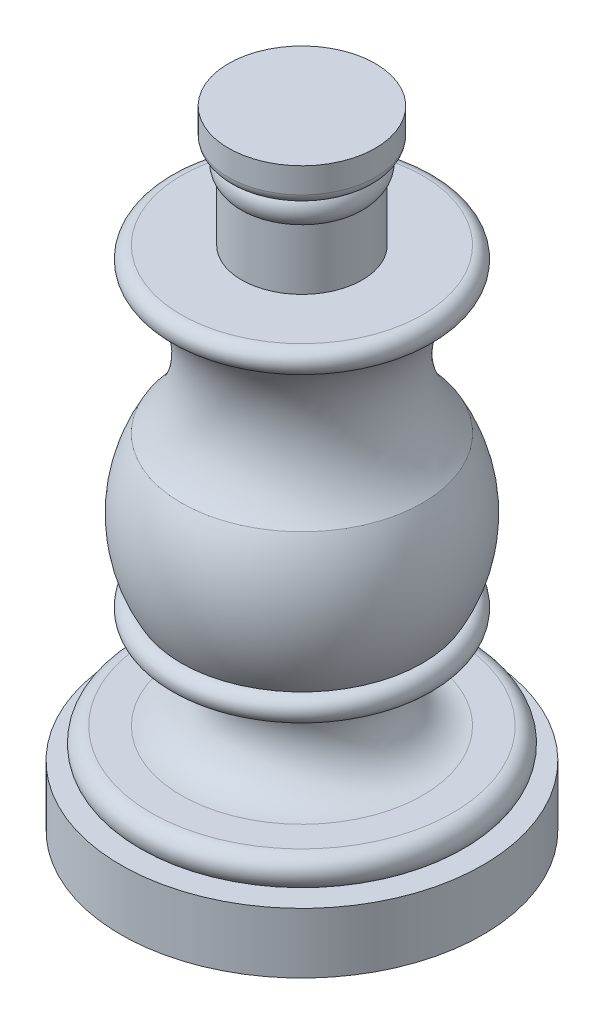
ISO-10303-21;
HEADER;
FILE_DESCRIPTION(('STEP AP214'),'2;1');
FILE_NAME('part.step','',(''),(''),'','','');
FILE_SCHEMA(('AUTOMOTIVE_DESIGN { 1 0 10303 214 1 1 1 1 }'));
ENDSEC;
DATA;
#1=APPLICATION_CONTEXT('core data for automotive mechanical design processes');
#2=APPLICATION_PROTOCOL_DEFINITION('international standard','automotive_design',2000,#1);
#3=PRODUCT_CONTEXT('',#1,'mechanical');
#4=PRODUCT('Part','Part','',(#3));
#5=PRODUCT_RELATED_PRODUCT_CATEGORY('part','',(#4));
#6=PRODUCT_DEFINITION_FORMATION('','',#4);
#7=PRODUCT_DEFINITION_CONTEXT('part definition',#1,'design');
#8=PRODUCT_DEFINITION('design','',#6,#7);
#9=PRODUCT_DEFINITION_SHAPE('','',#8);
#10=(LENGTH_UNIT() NAMED_UNIT(*) SI_UNIT(.MILLI.,.METRE.));
#11=(NAMED_UNIT(*) PLANE_ANGLE_UNIT() SI_UNIT($,.RADIAN.));
#12=(NAMED_UNIT(*) SI_UNIT($,.STERADIAN.) SOLID_ANGLE_UNIT());
#13=UNCERTAINTY_MEASURE_WITH_UNIT(LENGTH_MEASURE(1.E-05),#10,'distance_accuracy_value','');
#14=(GEOMETRIC_REPRESENTATION_CONTEXT(3) GLOBAL_UNCERTAINTY_ASSIGNED_CONTEXT((#13)) GLOBAL_UNIT_ASSIGNED_CONTEXT((#10,
#11,#12)) REPRESENTATION_CONTEXT('',''));
#15=CARTESIAN_POINT('',(0.,0.,0.));
#16=DIRECTION('',(0.,0.,1.));
#17=DIRECTION('',(1.,0.,0.));
#18=AXIS2_PLACEMENT_3D('',#15,#16,#17);
#19=CARTESIAN_POINT('',(0.,0.,0.));
#20=DIRECTION('',(0.,-1.,0.));
#21=DIRECTION('',(0.,0.,-1.));
#22=AXIS2_PLACEMENT_3D('',#19,#20,#21);
#23=PLANE('',#22);
#24=CARTESIAN_POINT('',(0.,0.,0.));
#25=DIRECTION('',(0.,-1.,0.));
#26=DIRECTION('',(0.,0.,-1.));
#27=AXIS2_PLACEMENT_3D('',#24,#25,#26);
#28=CIRCLE('',#27,30.);
#29=CARTESIAN_POINT('',(0.,0.,-30.));
#30=VERTEX_POINT('',#29);
#31=EDGE_CURVE('E10',#30,#30,#28,.T.);
#32=ORIENTED_EDGE('',*,*,#31,.T.);
#33=EDGE_LOOP('',(#32));
#34=FACE_BOUND('',#33,.T.);
#35=ADVANCED_FACE('F40',(#34),#23,.T.);
#36=CARTESIAN_POINT('',(0.,0.,0.));
#37=DIRECTION('',(0.,-1.,0.));
#38=DIRECTION('',(0.,0.,-1.));
#39=AXIS2_PLACEMENT_3D('',#36,#37,#38);
#40=CYLINDRICAL_SURFACE('',#39,30.);
#41=CARTESIAN_POINT('',(0.,10.,0.));
#42=DIRECTION('',(0.,-1.,0.));
#43=DIRECTION('',(0.,0.,-1.));
#44=AXIS2_PLACEMENT_3D('',#41,#42,#43);
#45=CIRCLE('',#44,30.);
#46=CARTESIAN_POINT('',(0.,10.,-30.));
#47=VERTEX_POINT('',#46);
#48=EDGE_CURVE('E43',#47,#47,#45,.T.);
#49=ORIENTED_EDGE('',*,*,#48,.T.);
#50=EDGE_LOOP('',(#49));
#51=FACE_BOUND('',#50,.T.);
#52=ORIENTED_EDGE('',*,*,#31,.F.);
#53=EDGE_LOOP('',(#52));
#54=FACE_BOUND('',#53,.T.);
#55=ADVANCED_FACE('F104',(#51,#54),#40,.T.);
#56=CARTESIAN_POINT('',(30.,10.,0.));
#57=DIRECTION('',(0.,1.,0.));
#58=DIRECTION('',(0.,0.,1.));
#59=AXIS2_PLACEMENT_3D('',#56,#57,#58);
#60=PLANE('',#59);
#61=CARTESIAN_POINT('',(0.,10.,0.));
#62=DIRECTION('',(0.,-1.,0.));
#63=DIRECTION('',(0.,0.,-1.));
#64=AXIS2_PLACEMENT_3D('',#61,#62,#63);
#65=CIRCLE('',#64,25.);
#66=CARTESIAN_POINT('',(0.,10.,-25.));
#67=VERTEX_POINT('',#66);
#68=EDGE_CURVE('E50',#67,#67,#65,.T.);
#69=ORIENTED_EDGE('',*,*,#68,.T.);
#70=EDGE_LOOP('',(#69));
#71=FACE_BOUND('',#70,.T.);
#72=ORIENTED_EDGE('',*,*,#48,.F.);
#73=EDGE_LOOP('',(#72));
#74=FACE_BOUND('',#73,.T.);
#75=ADVANCED_FACE('F108',(#71,#74),#60,.T.);
#76=CARTESIAN_POINT('',(0.,12.5,0.));
#77=DIRECTION('',(0.,-1.,0.));
#78=DIRECTION('',(0.,0.,-1.));
#79=AXIS2_PLACEMENT_3D('',#76,#77,#78);
#80=TOROIDAL_SURFACE('',#79,25.,2.5);
#81=CARTESIAN_POINT('',(0.,15.,0.));
#82=DIRECTION('',(0.,-1.,0.));
#83=DIRECTION('',(0.,0.,-1.));
#84=AXIS2_PLACEMENT_3D('',#81,#82,#83);
#85=CIRCLE('',#84,25.);
#86=CARTESIAN_POINT('',(0.,15.,-25.));
#87=VERTEX_POINT('',#86);
#88=EDGE_CURVE('E51',#87,#87,#85,.T.);
#89=ORIENTED_EDGE('',*,*,#88,.T.);
#90=EDGE_LOOP('',(#89));
#91=FACE_BOUND('',#90,.T.);
#92=ORIENTED_EDGE('',*,*,#68,.F.);
#93=EDGE_LOOP('',(#92));
#94=FACE_BOUND('',#93,.T.);
#95=ADVANCED_FACE('F114',(#91,#94),#80,.T.);
#96=CARTESIAN_POINT('',(20.,15.,0.));
#97=DIRECTION('',(0.,1.,0.));
#98=DIRECTION('',(0.,0.,1.));
#99=AXIS2_PLACEMENT_3D('',#96,#97,#98);
#100=PLANE('',#99);
#101=CARTESIAN_POINT('',(0.,15.,0.));
#102=DIRECTION('',(0.,-1.,0.));
#103=DIRECTION('',(0.,0.,-1.));
#104=AXIS2_PLACEMENT_3D('',#101,#102,#103);
#105=CIRCLE('',#104,20.);
#106=CARTESIAN_POINT('',(0.,15.,-20.));
#107=VERTEX_POINT('',#106);
#108=EDGE_CURVE('E57',#107,#107,#105,.T.);
#109=ORIENTED_EDGE('',*,*,#108,.T.);
#110=EDGE_LOOP('',(#109));
#111=FACE_BOUND('',#110,.T.);
#112=ORIENTED_EDGE('',*,*,#88,.F.);
#113=EDGE_LOOP('',(#112));
#114=FACE_BOUND('',#113,.T.);
#115=ADVANCED_FACE('F118',(#111,#114),#100,.T.);
#116=CARTESIAN_POINT('',(0.,22.5,0.));
#117=DIRECTION('',(0.,-1.,0.));
#118=DIRECTION('',(0.,0.,-1.));
#119=AXIS2_PLACEMENT_3D('',#116,#117,#118);
#120=TOROIDAL_SURFACE('',#119,20.,7.5);
#121=CARTESIAN_POINT('',(0.,30.,0.));
#122=DIRECTION('',(0.,-1.,0.));
#123=DIRECTION('',(0.,0.,-1.));
#124=AXIS2_PLACEMENT_3D('',#121,#122,#123);
#125=CIRCLE('',#124,20.);
#126=CARTESIAN_POINT('',(0.,30.,-20.));
#127=VERTEX_POINT('',#126);
#128=EDGE_CURVE('E56',#127,#127,#125,.T.);
#129=ORIENTED_EDGE('',*,*,#128,.T.);
#130=EDGE_LOOP('',(#129));
#131=FACE_BOUND('',#130,.T.);
#132=ORIENTED_EDGE('',*,*,#108,.F.);
#133=EDGE_LOOP('',(#132));
#134=FACE_BOUND('',#133,.T.);
#135=ADVANCED_FACE('F122',(#131,#134),#120,.F.);
#136=CARTESIAN_POINT('',(0.,32.,0.));
#137=DIRECTION('',(0.,-1.,0.));
#138=DIRECTION('',(0.,0.,-1.));
#139=AXIS2_PLACEMENT_3D('',#136,#137,#138);
#140=TOROIDAL_SURFACE('',#139,20.,2.);
#141=CARTESIAN_POINT('',(0.,34.,0.));
#142=DIRECTION('',(0.,-1.,0.));
#143=DIRECTION('',(0.,0.,-1.));
#144=AXIS2_PLACEMENT_3D('',#141,#142,#143);
#145=CIRCLE('',#144,20.);
#146=CARTESIAN_POINT('',(20.,34.,0.));
#147=VERTEX_POINT('',#146);
#148=EDGE_CURVE('E65',#147,#147,#145,.T.);
#149=ORIENTED_EDGE('',*,*,#148,.T.);
#150=EDGE_LOOP('',(#149));
#151=FACE_BOUND('',#150,.T.);
#152=ORIENTED_EDGE('',*,*,#128,.F.);
#153=EDGE_LOOP('',(#152));
#154=FACE_BOUND('',#153,.T.);
#155=ADVANCED_FACE('F126',(#151,#154),#140,.T.);
#156=CARTESIAN_POINT('',(0.,45.5,0.));
#157=DIRECTION('',(0.,-1.,0.));
#158=DIRECTION('',(1.,0.,0.));
#159=AXIS2_PLACEMENT_3D('',#156,#157,#158);
#160=SPHERICAL_SURFACE('',#159,23.0705439901187);
#161=CARTESIAN_POINT('',(0.,57.,0.));
#162=DIRECTION('',(0.,-1.,0.));
#163=DIRECTION('',(0.,0.,-1.));
#164=AXIS2_PLACEMENT_3D('',#161,#162,#163);
#165=CIRCLE('',#164,20.);
#166=CARTESIAN_POINT('',(20.,57.,0.));
#167=VERTEX_POINT('',#166);
#168=EDGE_CURVE('E63',#167,#167,#165,.T.);
#169=CARTESIAN_POINT('',(20.,57.,0.));
#170=CARTESIAN_POINT('',(20.1250241745514,56.7825697856751,0.));
#171=CARTESIAN_POINT('',(20.2464999297138,56.5630993319941,0.));
#172=CARTESIAN_POINT('',(20.4822314536365,56.1203146036134,0.));
#173=CARTESIAN_POINT('',(20.5964872223969,55.8970003289136,0.));
#174=CARTESIAN_POINT('',(20.8176556258917,55.4467646161882,0.));
#175=CARTESIAN_POINT('',(20.9245682606261,55.2198431781625,0.));
#176=CARTESIAN_POINT('',(21.1309371164233,54.7626347286063,0.));
#177=CARTESIAN_POINT('',(21.230393337486,54.5323477170758,0.));
#178=CARTESIAN_POINT('',(21.4217434657383,54.0686529964927,0.));
#179=CARTESIAN_POINT('',(21.5136373729279,53.8352452874402,0.));
#180=CARTESIAN_POINT('',(21.6897651643995,53.3655574456856,0.));
#181=CARTESIAN_POINT('',(21.7739990486815,53.1292773129836,0.));
#182=CARTESIAN_POINT('',(21.9347171930767,52.6540959318972,0.));
#183=CARTESIAN_POINT('',(22.0112014531899,52.4151946835127,0.));
#184=CARTESIAN_POINT('',(22.1563390012529,51.935025172548,0.));
#185=CARTESIAN_POINT('',(22.2249922892027,51.6937569099677,0.));
#186=CARTESIAN_POINT('',(22.354394871286,51.2091099881898,0.));
#187=CARTESIAN_POINT('',(22.4151441654194,50.9657313289923,0.));
#188=CARTESIAN_POINT('',(22.5286741458289,50.4771224766253,0.));
#189=CARTESIAN_POINT('',(22.5814548321051,50.2318922834559,0.));
#190=CARTESIAN_POINT('',(22.678991458131,49.7398411950116,0.));
#191=CARTESIAN_POINT('',(22.7237473978807,49.4930202997368,0.));
#192=CARTESIAN_POINT('',(22.8051869275249,48.9980503308809,0.));
#193=CARTESIAN_POINT('',(22.8418705174195,48.7499012572997,0.));
#194=CARTESIAN_POINT('',(22.9071263299277,48.2525388683004,0.));
#195=CARTESIAN_POINT('',(22.9356985525415,48.0033255528821,0.));
#196=CARTESIAN_POINT('',(22.984701240484,47.5040997486293,0.));
#197=CARTESIAN_POINT('',(23.0051317058127,47.2540872597948,0.));
#198=CARTESIAN_POINT('',(23.0378291489208,46.7535290271469,0.));
#199=CARTESIAN_POINT('',(23.0500961267002,46.5029832833335,0.));
#200=CARTESIAN_POINT('',(23.0664535472991,46.0016250263468,0.));
#201=CARTESIAN_POINT('',(23.0705439901187,45.7508125131734,0.));
#202=CARTESIAN_POINT('',(23.0705439901187,45.2491874868266,0.));
#203=CARTESIAN_POINT('',(23.0664535472991,44.9983749736532,0.));
#204=CARTESIAN_POINT('',(23.0500961267002,44.4970167166665,0.));
#205=CARTESIAN_POINT('',(23.0378291489208,44.2464709728532,0.));
#206=CARTESIAN_POINT('',(23.0051317058127,43.7459127402053,0.));
#207=CARTESIAN_POINT('',(22.984701240484,43.4959002513707,0.));
#208=CARTESIAN_POINT('',(22.9356985525415,42.9966744471179,0.));
#209=CARTESIAN_POINT('',(22.9071263299277,42.7474611316996,0.));
#210=CARTESIAN_POINT('',(22.8418705174195,42.2500987427003,0.));
#211=CARTESIAN_POINT('',(22.8051869275249,42.0019496691192,0.));
#212=CARTESIAN_POINT('',(22.7237473978807,41.5069797002632,0.));
#213=CARTESIAN_POINT('',(22.678991458131,41.2601588049884,0.));
#214=CARTESIAN_POINT('',(22.5814548321051,40.7681077165441,0.));
#215=CARTESIAN_POINT('',(22.5286741458289,40.5228775233747,0.));
#216=CARTESIAN_POINT('',(22.4151441654194,40.0342686710077,0.));
#217=CARTESIAN_POINT('',(22.354394871286,39.7908900118102,0.));
#218=CARTESIAN_POINT('',(22.2249922892027,39.3062430900323,0.));
#219=CARTESIAN_POINT('',(22.1563390012529,39.064974827452,0.));
#220=CARTESIAN_POINT('',(22.0112014531899,38.5848053164873,0.));
#221=CARTESIAN_POINT('',(21.9347171930767,38.3459040681028,0.));
#222=CARTESIAN_POINT('',(21.7739990486815,37.8707226870164,0.));
#223=CARTESIAN_POINT('',(21.6897651643995,37.6344425543144,0.));
#224=CARTESIAN_POINT('',(21.5136373729279,37.1647547125599,0.));
#225=CARTESIAN_POINT('',(21.4217434657383,36.9313470035073,0.));
#226=CARTESIAN_POINT('',(21.230393337486,36.4676522829242,0.));
#227=CARTESIAN_POINT('',(21.1309371164233,36.2373652713937,0.));
#228=CARTESIAN_POINT('',(20.9245682606261,35.7801568218375,0.));
#229=CARTESIAN_POINT('',(20.8176556258917,35.5532353838119,0.));
#230=CARTESIAN_POINT('',(20.5964872223969,35.1029996710864,0.));
#231=CARTESIAN_POINT('',(20.4822314536365,34.8796853963866,0.));
#232=CARTESIAN_POINT('',(20.2464999297138,34.4369006680059,0.));
#233=CARTESIAN_POINT('',(20.1250241745514,34.217430214325,0.));
#234=CARTESIAN_POINT('',(20.,34.,0.));
#235=B_SPLINE_CURVE_WITH_KNOTS('',3,(#169,#170,#171,#172,#173,#174,#175,#176,#177,#178,#179,
#180,#181,#182,#183,#184,#185,#186,#187,#188,#189,#190,#191,#192,#193,#194,#195,#196,#197,#198,
#199,#200,#201,#202,#203,#204,#205,#206,#207,#208,#209,#210,#211,#212,#213,#214,#215,#216,#217,
#218,#219,#220,#221,#222,#223,#224,#225,#226,#227,#228,#229,#230,#231,#232,#233,#234),
.UNSPECIFIED.,.F.,.F.,(4,2,2,2,2,2,2,2,2,2,2,2,2,2,2,2,2,2,2,2,2,2,2,2,2,2,2,2,2,2,2,2,4),(0.,
0.752404195567785,1.50480839113557,2.25721258670336,3.00961678227114,3.76202097783892,
4.51442517340671,5.2668293689745,6.01923356454228,6.77163776011007,7.52404195567786,
8.27644615124564,9.02885034681342,9.78125454238121,10.533658737949,11.2860629335168,
12.0384671290846,12.7908713246524,13.5432755202201,14.2956797157879,15.0480839113557,
15.8004881069235,16.5528923024913,17.3052964980591,18.0577006936268,18.8101048891946,
19.5625090847624,20.3149132803302,21.067317475898,21.8197216714658,22.5721258670336,
23.3245300626013,24.0769342581691),.UNSPECIFIED.);
#236=EDGE_CURVE('BSEAM135',#167,#147,#235,.T.);
#237=ORIENTED_EDGE('',*,*,#168,.T.);
#238=ORIENTED_EDGE('',*,*,#148,.F.);
#239=ORIENTED_EDGE('',*,*,#236,.T.);
#240=ORIENTED_EDGE('',*,*,#236,.F.);
#241=EDGE_LOOP('',(#237,#239,#238,#240));
#242=FACE_BOUND('',#241,.T.);
#243=ADVANCED_FACE('F135',(#242),#160,.T.);
#244=CARTESIAN_POINT('',(0.,68.5,0.));
#245=DIRECTION('',(0.,-1.,0.));
#246=DIRECTION('',(0.,0.,-1.));
#247=AXIS2_PLACEMENT_3D('',#244,#245,#246);
#248=TOROIDAL_SURFACE('',#247,31.5,16.2634559672906);
#249=CARTESIAN_POINT('',(0.,80.,0.));
#250=DIRECTION('',(0.,-1.,0.));
#251=DIRECTION('',(0.,0.,-1.));
#252=AXIS2_PLACEMENT_3D('',#249,#250,#251);
#253=CIRCLE('',#252,20.);
#254=CARTESIAN_POINT('',(0.,80.,-20.));
#255=VERTEX_POINT('',#254);
#256=EDGE_CURVE('E68',#255,#255,#253,.T.);
#257=ORIENTED_EDGE('',*,*,#256,.T.);
#258=EDGE_LOOP('',(#257));
#259=FACE_BOUND('',#258,.T.);
#260=ORIENTED_EDGE('',*,*,#168,.F.);
#261=EDGE_LOOP('',(#260));
#262=FACE_BOUND('',#261,.T.);
#263=ADVANCED_FACE('F136',(#259,#262),#248,.F.);
#264=CARTESIAN_POINT('',(0.,82.,0.));
#265=DIRECTION('',(0.,-1.,0.));
#266=DIRECTION('',(0.,0.,-1.));
#267=AXIS2_PLACEMENT_3D('',#264,#265,#266);
#268=TOROIDAL_SURFACE('',#267,20.,2.);
#269=CARTESIAN_POINT('',(0.,84.,0.));
#270=DIRECTION('',(0.,-1.,0.));
#271=DIRECTION('',(0.,0.,-1.));
#272=AXIS2_PLACEMENT_3D('',#269,#270,#271);
#273=CIRCLE('',#272,20.);
#274=CARTESIAN_POINT('',(0.,84.,-20.));
#275=VERTEX_POINT('',#274);
#276=EDGE_CURVE('E72',#275,#275,#273,.T.);
#277=ORIENTED_EDGE('',*,*,#276,.T.);
#278=EDGE_LOOP('',(#277));
#279=FACE_BOUND('',#278,.T.);
#280=ORIENTED_EDGE('',*,*,#256,.F.);
#281=EDGE_LOOP('',(#280));
#282=FACE_BOUND('',#281,.T.);
#283=ADVANCED_FACE('F139',(#279,#282),#268,.T.);
#284=CARTESIAN_POINT('',(20.,84.,0.));
#285=DIRECTION('',(0.,1.,0.));
#286=DIRECTION('',(0.,0.,1.));
#287=AXIS2_PLACEMENT_3D('',#284,#285,#286);
#288=PLANE('',#287);
#289=CARTESIAN_POINT('',(0.,84.,0.));
#290=DIRECTION('',(0.,-1.,0.));
#291=DIRECTION('',(0.,0.,-1.));
#292=AXIS2_PLACEMENT_3D('',#289,#290,#291);
#293=CIRCLE('',#292,10.);
#294=CARTESIAN_POINT('',(0.,84.,-10.));
#295=VERTEX_POINT('',#294);
#296=EDGE_CURVE('E74',#295,#295,#293,.T.);
#297=ORIENTED_EDGE('',*,*,#296,.T.);
#298=EDGE_LOOP('',(#297));
#299=FACE_BOUND('',#298,.T.);
#300=ORIENTED_EDGE('',*,*,#276,.F.);
#301=EDGE_LOOP('',(#300));
#302=FACE_BOUND('',#301,.T.);
#303=ADVANCED_FACE('F145',(#299,#302),#288,.T.);
#304=CARTESIAN_POINT('',(0.,0.,0.));
#305=DIRECTION('',(0.,-1.,0.));
#306=DIRECTION('',(0.,0.,-1.));
#307=AXIS2_PLACEMENT_3D('',#304,#305,#306);
#308=CYLINDRICAL_SURFACE('',#307,10.);
#309=CARTESIAN_POINT('',(0.,94.,0.));
#310=DIRECTION('',(0.,-1.,0.));
#311=DIRECTION('',(0.,0.,-1.));
#312=AXIS2_PLACEMENT_3D('',#309,#310,#311);
#313=CIRCLE('',#312,10.);
#314=CARTESIAN_POINT('',(0.,94.,-10.));
#315=VERTEX_POINT('',#314);
#316=EDGE_CURVE('E80',#315,#315,#313,.T.);
#317=ORIENTED_EDGE('',*,*,#316,.T.);
#318=EDGE_LOOP('',(#317));
#319=FACE_BOUND('',#318,.T.);
#320=ORIENTED_EDGE('',*,*,#296,.F.);
#321=EDGE_LOOP('',(#320));
#322=FACE_BOUND('',#321,.T.);
#323=ADVANCED_FACE('F146',(#319,#322),#308,.T.);
#324=CARTESIAN_POINT('',(0.,96.,0.));
#325=DIRECTION('',(0.,-1.,0.));
#326=DIRECTION('',(0.,0.,-1.));
#327=AXIS2_PLACEMENT_3D('',#324,#325,#326);
#328=TOROIDAL_SURFACE('',#327,7.99999999999996,2.82842712474622);
#329=CARTESIAN_POINT('',(0.,98.,0.));
#330=DIRECTION('',(0.,-1.,0.));
#331=DIRECTION('',(0.,0.,-1.));
#332=AXIS2_PLACEMENT_3D('',#329,#330,#331);
#333=CIRCLE('',#332,10.);
#334=CARTESIAN_POINT('',(0.,98.,-10.));
#335=VERTEX_POINT('',#334);
#336=EDGE_CURVE('E78',#335,#335,#333,.T.);
#337=ORIENTED_EDGE('',*,*,#336,.T.);
#338=EDGE_LOOP('',(#337));
#339=FACE_BOUND('',#338,.T.);
#340=ORIENTED_EDGE('',*,*,#316,.F.);
#341=EDGE_LOOP('',(#340));
#342=FACE_BOUND('',#341,.T.);
#343=ADVANCED_FACE('F155',(#339,#342),#328,.T.);
#344=CARTESIAN_POINT('',(10.3530166058249,98.,0.));
#345=DIRECTION('',(0.,-1.,0.));
#346=DIRECTION('',(0.,0.,-1.));
#347=AXIS2_PLACEMENT_3D('',#344,#345,#346);
#348=PLANE('',#347);
#349=CARTESIAN_POINT('',(0.,98.,0.));
#350=DIRECTION('',(0.,-1.,0.));
#351=DIRECTION('',(0.,0.,-1.));
#352=AXIS2_PLACEMENT_3D('',#349,#350,#351);
#353=CIRCLE('',#352,10.3530166058249);
#354=CARTESIAN_POINT('',(0.,98.,-10.3530166058249));
#355=VERTEX_POINT('',#354);
#356=EDGE_CURVE('E83',#355,#355,#353,.T.);
#357=ORIENTED_EDGE('',*,*,#356,.T.);
#358=EDGE_LOOP('',(#357));
#359=FACE_BOUND('',#358,.T.);
#360=ORIENTED_EDGE('',*,*,#336,.F.);
#361=EDGE_LOOP('',(#360));
#362=FACE_BOUND('',#361,.T.);
#363=ADVANCED_FACE('F156',(#359,#362),#348,.T.);
#364=CARTESIAN_POINT('',(0.,99.9921959790651,0.));
#365=DIRECTION('',(0.,-1.,0.));
#366=DIRECTION('',(0.,0.,-1.));
#367=AXIS2_PLACEMENT_3D('',#364,#365,#366);
#368=TOROIDAL_SURFACE('',#367,10.1765083029125,2.);
#369=CARTESIAN_POINT('',(0.,99.8156876761526,0.));
#370=DIRECTION('',(0.,-1.,0.));
#371=DIRECTION('',(0.,0.,-1.));
#372=AXIS2_PLACEMENT_3D('',#369,#370,#371);
#373=CIRCLE('',#372,12.1687042819775);
#374=CARTESIAN_POINT('',(0.,99.8156876761526,-12.1687042819775));
#375=VERTEX_POINT('',#374);
#376=EDGE_CURVE('E88',#375,#375,#373,.T.);
#377=ORIENTED_EDGE('',*,*,#376,.T.);
#378=EDGE_LOOP('',(#377));
#379=FACE_BOUND('',#378,.T.);
#380=ORIENTED_EDGE('',*,*,#356,.F.);
#381=EDGE_LOOP('',(#380));
#382=FACE_BOUND('',#381,.T.);
#383=ADVANCED_FACE('F105',(#379,#382),#368,.T.);
#384=CARTESIAN_POINT('',(0.,0.,0.));
#385=DIRECTION('',(0.,-1.,0.));
#386=DIRECTION('',(0.,0.,-1.));
#387=AXIS2_PLACEMENT_3D('',#384,#385,#386);
#388=CYLINDRICAL_SURFACE('',#387,12.1687042819775);
#389=CARTESIAN_POINT('',(0.,104.,0.));
#390=DIRECTION('',(0.,-1.,0.));
#391=DIRECTION('',(0.,0.,-1.));
#392=AXIS2_PLACEMENT_3D('',#389,#390,#391);
#393=CIRCLE('',#392,12.1687042819775);
#394=CARTESIAN_POINT('',(0.,104.,-12.1687042819775));
#395=VERTEX_POINT('',#394);
#396=EDGE_CURVE('E90',#395,#395,#393,.T.);
#397=ORIENTED_EDGE('',*,*,#396,.T.);
#398=EDGE_LOOP('',(#397));
#399=FACE_BOUND('',#398,.T.);
#400=ORIENTED_EDGE('',*,*,#376,.F.);
#401=EDGE_LOOP('',(#400));
#402=FACE_BOUND('',#401,.T.);
#403=ADVANCED_FACE('F91',(#399,#402),#388,.T.);
#404=CARTESIAN_POINT('',(0.,104.,0.));
#405=DIRECTION('',(0.,1.,0.));
#406=DIRECTION('',(0.,0.,1.));
#407=AXIS2_PLACEMENT_3D('',#404,#405,#406);
#408=PLANE('',#407);
#409=ORIENTED_EDGE('',*,*,#396,.F.);
#410=EDGE_LOOP('',(#409));
#411=FACE_BOUND('',#410,.T.);
#412=ADVANCED_FACE('F96',(#411),#408,.T.);
#413=CLOSED_SHELL('',(#35,#55,#75,#95,#115,#135,#155,#243,#263,#283,#303,#323,#343,#363,#383,
#403,#412));
#414=MANIFOLD_SOLID_BREP('B2',#413);
#415=ADVANCED_BREP_SHAPE_REPRESENTATION('',(#18,#414),#14);
#416=SHAPE_DEFINITION_REPRESENTATION(#9,#415);
ENDSEC;
END-ISO-10303-21;
